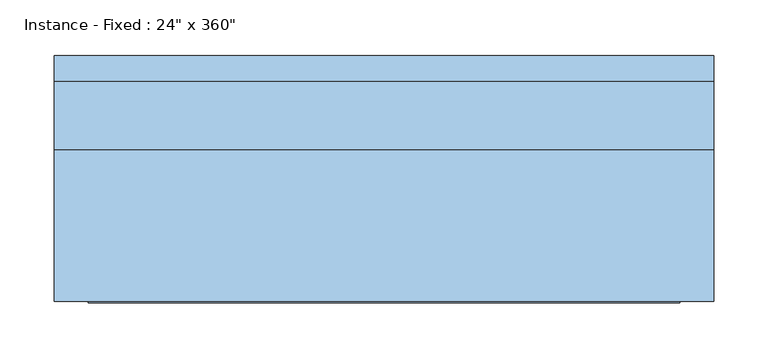
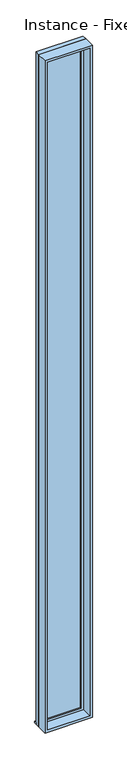
"""IFC4 building model written with IfcOpenShell, lengths in millimetres: window geometry."""

from ifc_helpers import new_model, si_unit, frame, origin, place, context, project, spatial, polyline, outline, extrude, source, transform, mapped, element, save


def window_44a3cfc2(model_context):
    return source(origin(), model_context, "Body", "SweptSolid", [
        extrude(outline(polyline([(-342.9, 127.0), (266.7, 127.0), (266.7, 101.6), (-342.9, 101.6), (-342.9, 127.0)])), frame((0.0, 0.0, 6096.0), z_axis=(0.0, 0.0, 1.0), x_axis=(1.0, 0.0, 0.0)), (0.0, 0.0, 1.0), 19.05),
        extrude(outline(polyline([(203.2, 53.975), (-279.4, 53.975), (-279.4, 66.675), (203.2, 66.675), (203.2, 53.975)])), frame((0.0, 0.0, 6159.5), z_axis=(0.0, 0.0, 1.0), x_axis=(1.0, 0.0, 0.0)), (0.0, 0.0, 1.0), 9017.0),
        extrude(outline(polyline([(15220.95, -323.85), (6115.05, -323.85), (6115.05, 247.65), (15220.95, 247.65), (15220.95, -323.85)]), holes=[polyline([(15176.5, -279.4), (15176.5, 203.2), (6159.5, 203.2), (6159.5, -279.4), (15176.5, -279.4)])]), frame((0.0, 38.1, 0.0), z_axis=(0.0, 1.0, 0.0), x_axis=(0.0, 0.0, 1.0)), (0.0, 0.0, 1.0), 44.45),
        extrude(outline(polyline([(15240.0, -342.9), (6096.0, -342.9), (6096.0, 266.7), (15240.0, 266.7), (15240.0, -342.9)]), holes=[polyline([(15208.25, -311.15), (15208.25, 234.95), (6127.75, 234.95), (6127.75, -311.15), (15208.25, -311.15)])]), frame((0.0, -101.6, 0.0), z_axis=(0.0, 1.0, 0.0), x_axis=(0.0, 0.0, 1.0)), (0.0, 0.0, 1.0), 139.7),
        extrude(outline(polyline([(15240.0, 266.7), (15240.0, -342.9), (6096.0, -342.9), (6096.0, 266.7), (15240.0, 266.7)]), holes=[polyline([(15220.95, 247.65), (6115.05, 247.65), (6115.05, -323.85), (15220.95, -323.85), (15220.95, 247.65)])]), frame((0.0, 38.1, 0.0), z_axis=(0.0, 1.0, 0.0), x_axis=(0.0, 0.0, 1.0)), (0.0, 0.0, 1.0), 63.5),
    ])


if __name__ == "__main__":
    model = new_model("IFC4")
    model_context = context("Model", 3, world=origin())
    ifc_project = project(units=[si_unit("LENGTHUNIT", "METRE", prefix="MILLI")], contexts=[model_context])
    site = spatial("IfcSite", under=ifc_project)
    building = spatial("IfcBuilding", under=site)
    placement = place(None, origin())
    window_shape = window_44a3cfc2(model_context)
    element("IfcWindow", 1, ObjectType="Instance - Fixed : 24\" x 360\"", at=placement, inside=building, context=model_context, shape_type="MappedRepresentation", body=[
        mapped(window_shape, transform((0.0, 0.0, 0.0), x_axis=(1.0, 0.0, 0.0), y_axis=(0.0, 1.0, 0.0), z_axis=(0.0, 0.0, 1.0))),
    ])
    save(model, "model.ifc")

# Revit data of these elements
# Type "Instance - Fixed : 24\" x 360\""
#   Type Mark = "10"
#   Construction Type Id = "GSP4R"
#   Assembly Code = "B2020100"
#   Analytic Construction = "1/8 in Pilkington single glazing"
#   Visual Light Transmittance = 0.9
#   Thermal Resistance (R) = 0.8466 (h·ft²·°F)/BTU
#   Solar Heat Gain Coefficient = 0.86
#   Heat Transfer Coefficient (U) = 1.1812 BTU/(h·ft²·°F)
#   Height [instance default] = 4' - 0"
#   Default Sill Height = 20' - 0"
#   Width [instance default] = 2' - 0"
#   Window Inset = 0' - 0 3/4"
#   Define Thermal Properties by = 1
#   Glass Pane Material = Glass
#   Sash Material = Default Roof
#   Wall Closure = (empty or 0)
# Element 1 (IfcWindow, "Instance - Fixed : 24\" x 360\"")
#   Height = 30' - 0"
#   Materials on its faces: "Default Roof", "Glass"
# Materials
#   "Glass": class "Glass", colour RGB 0 128 192, transparency 0.75, Description = "Soda Lime Glass", Cost = 0
#   "Default Roof": colour RGB 88 101 114, transparency 0
